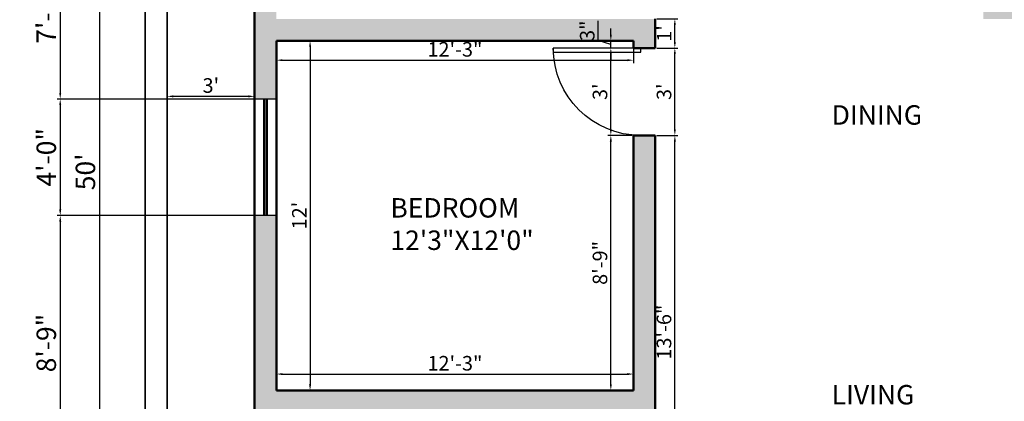
# Model space of a CAD drawing. Units: inches. Extents: x 2442 to 3851, y 589 to 2836.
# Tile 14 of 22: x 2442 to 2847, y 2397 to 2554. Entities that reach past the tile are written whole.
import ezdxf

# ---------------------------------------------------------------- set-up
doc = ezdxf.new("R2010")
doc.units = ezdxf.units.IN
for name, color, linetype, lineweight in [('A-ANNO-DIMS', 2, 'Continuous', 18), ('A-AREA-IDEN', 7, 'Continuous', 18), ('A-DOOR', 4, 'Continuous', 25), ('A-GLAZ', 1, 'Continuous', 25), ('A-WALL', 7, 'Continuous', 50), ('A-WALL-PATT', 8, 'Continuous', 13), ('C-PROP', 7, 'Continuous', 35)]:
    doc.layers.add(name, color=color, linetype=linetype, lineweight=lineweight)
doc.styles.get("Standard").update_dxf_attribs({"font": 'arial.ttf'})
doc.dimstyles.new('ISO-25', dxfattribs={"dimtxt": 8, "dimasz": 2.5, "dimexe": 1.25, "dimexo": 0.625, "dimtad": 1, "dimlunit": 3, "dimtxsty": 'Standard', "dimcen": 2.5, "dimadec": 0, "dimazin": 0, "dimtfac": 1, "dimtmove": 0, "dimatfit": 3, "dimfxl": 1, "dimarcsym": 0})

# ---------------------------------------------------------------- blocks, each defined once
blk = doc.blocks.new('*U23')
for p, q in [((0, 0), (0, -6)), ((36, 0), (36, -6))]:
    blk.add_line(p, q)
blk.add_lwpolyline([(0, 0), (0, 36), (1.75, 36), (1.75, 0)], close=True)
blk.add_arc((0, 0), 36, 0, 90)
blk = doc.blocks.new('*D36')
at = {"layer": 'A-ANNO-DIMS', "color": 0, "lineweight": -2, "transparency": 16777216}
for p, q in [((2492.97, 2791.21), (2473.47, 2791.21)), ((2474.72, 2788.71), (2474.72, 2193.71)), ((2492.97, 2191.21), (2473.47, 2191.21))]:
    blk.add_line(p, q, dxfattribs=at)
at = {"layer": 'A-ANNO-DIMS', "color": 0, "transparency": 16777216}
for points in [[(2474.3, 2788.71), (2475.14, 2788.71), (2474.72, 2791.21)], [(2474.3, 2193.71), (2475.14, 2193.71), (2474.72, 2191.21)]]:
    blk.add_solid(points, dxfattribs=at)
at = {"layer": 'Defpoints', "color": 0, "transparency": 16777216}
for p in [(2493.6, 2791.21), (2474.72, 2191.21), (2493.6, 2191.21)]:
    blk.add_point(p, dxfattribs=at)
at = {"layer": 'A-ANNO-DIMS', "color": 0, "transparency": 16777216, "insert": (2470.01, 2491.21), "char_height": 8, "attachment_point": 5, "rotation": 90}
blk.add_mtext("50'", dxfattribs=at)
blk = doc.blocks.new('*D41')
at = {"layer": 'A-ANNO-DIMS', "color": 0, "lineweight": -2, "transparency": 16777216}
for p, q in [((2502.6, 2521.83), (2502.6, 2523.56)), ((2536.1, 2522.31), (2505.1, 2522.31)), ((2538.6, 2521.83), (2538.6, 2523.56))]:
    blk.add_line(p, q, dxfattribs=at)
at = {"layer": 'A-ANNO-DIMS', "color": 0, "transparency": 16777216}
for points in [[(2505.1, 2522.73), (2505.1, 2521.89), (2502.6, 2522.31)], [(2536.1, 2522.73), (2536.1, 2521.89), (2538.6, 2522.31)]]:
    blk.add_solid(points, dxfattribs=at)
at = {"layer": 'Defpoints', "color": 0, "transparency": 16777216}
for p in [(2502.6, 2522.31), (2502.6, 2521.21), (2538.6, 2521.21)]:
    blk.add_point(p, dxfattribs=at)
at = {"layer": 'A-ANNO-DIMS', "color": 0, "transparency": 16777216, "insert": (2520.6, 2526), "char_height": 6, "attachment_point": 5}
blk.add_mtext("3'", dxfattribs=at)
blk = doc.blocks.new('*D56')
at = {"layer": 'A-ANNO-DIMS', "color": 0, "lineweight": -2, "transparency": 16777216}
for p, q in [((2548.22, 2545.21), (2562.71, 2545.21)), ((2561.46, 2542.71), (2561.46, 2403.71)), ((2548.22, 2401.21), (2562.71, 2401.21))]:
    blk.add_line(p, q, dxfattribs=at)
at = {"layer": 'A-ANNO-DIMS', "color": 0, "transparency": 16777216}
for points in [[(2561.05, 2542.71), (2561.88, 2542.71), (2561.46, 2545.21)], [(2561.05, 2403.71), (2561.88, 2403.71), (2561.46, 2401.21)]]:
    blk.add_solid(points, dxfattribs=at)
at = {"layer": 'Defpoints', "color": 0, "transparency": 16777216}
for p in [(2547.6, 2545.21), (2547.6, 2401.21), (2561.46, 2401.21)]:
    blk.add_point(p, dxfattribs=at)
at = {"layer": 'A-ANNO-DIMS', "color": 0, "transparency": 16777216, "insert": (2557.83, 2473.21), "char_height": 6, "attachment_point": 5, "rotation": 90}
blk.add_mtext("12'", dxfattribs=at)
blk = doc.blocks.new('*D57')
at = {"layer": 'A-ANNO-DIMS', "color": 0, "lineweight": -2, "transparency": 16777216}
for p, q in [((2547.6, 2401.83), (2547.6, 2409.17)), ((2550.1, 2407.92), (2692.1, 2407.92)), ((2694.6, 2401.83), (2694.6, 2409.17))]:
    blk.add_line(p, q, dxfattribs=at)
at = {"layer": 'A-ANNO-DIMS', "color": 0, "transparency": 16777216}
for points in [[(2550.1, 2408.34), (2550.1, 2407.51), (2547.6, 2407.92)], [(2692.1, 2408.34), (2692.1, 2407.51), (2694.6, 2407.92)]]:
    blk.add_solid(points, dxfattribs=at)
at = {"layer": 'Defpoints', "color": 0, "transparency": 16777216}
for p in [(2694.6, 2407.92), (2547.6, 2401.21), (2694.6, 2401.21)]:
    blk.add_point(p, dxfattribs=at)
at = {"layer": 'A-ANNO-DIMS', "color": 0, "transparency": 16777216, "insert": (2621.1, 2411.61), "char_height": 6, "attachment_point": 5}
blk.add_mtext('12\'-3"', dxfattribs=at)
blk = doc.blocks.new('*D73')
at = {"layer": 'A-ANNO-DIMS', "color": 0, "lineweight": -2, "transparency": 16777216}
for p, q in [((2693.97, 2506.21), (2684.03, 2506.21)), ((2685.28, 2403.71), (2685.28, 2503.71)), ((2693.97, 2401.21), (2684.03, 2401.21))]:
    blk.add_line(p, q, dxfattribs=at)
at = {"layer": 'A-ANNO-DIMS', "color": 0, "transparency": 16777216}
for points in [[(2684.87, 2503.71), (2685.7, 2503.71), (2685.28, 2506.21)], [(2684.87, 2403.71), (2685.7, 2403.71), (2685.28, 2401.21)]]:
    blk.add_solid(points, dxfattribs=at)
at = {"layer": 'Defpoints', "color": 0, "transparency": 16777216}
for p in [(2685.28, 2506.21), (2694.6, 2506.21), (2694.6, 2401.21)]:
    blk.add_point(p, dxfattribs=at)
at = {"layer": 'A-ANNO-DIMS', "color": 0, "transparency": 16777216, "insert": (2681.59, 2453.71), "char_height": 6, "attachment_point": 5, "rotation": 90}
blk.add_mtext('8\'-9"', dxfattribs=at)
blk = doc.blocks.new('*D74')
at = {"layer": 'A-ANNO-DIMS', "color": 0, "lineweight": -2, "transparency": 16777216}
for p, q in [((2693.97, 2542.21), (2684.03, 2542.21)), ((2685.28, 2508.71), (2685.28, 2539.71)), ((2693.97, 2506.21), (2684.03, 2506.21))]:
    blk.add_line(p, q, dxfattribs=at)
at = {"layer": 'A-ANNO-DIMS', "color": 0, "transparency": 16777216}
for points in [[(2684.87, 2539.71), (2685.7, 2539.71), (2685.28, 2542.21)], [(2684.87, 2508.71), (2685.7, 2508.71), (2685.28, 2506.21)]]:
    blk.add_solid(points, dxfattribs=at)
at = {"layer": 'Defpoints', "color": 0, "transparency": 16777216}
for p in [(2685.28, 2542.21), (2694.6, 2542.21), (2694.6, 2506.21)]:
    blk.add_point(p, dxfattribs=at)
at = {"layer": 'A-ANNO-DIMS', "color": 0, "transparency": 16777216, "insert": (2681.59, 2524.21), "char_height": 6, "attachment_point": 5, "rotation": 90}
blk.add_mtext("3'", dxfattribs=at)
blk = doc.blocks.new('*D75')
at = {"layer": 'A-ANNO-DIMS', "color": 0, "lineweight": -2, "transparency": 16777216}
for p, q in [((2680.03, 2545.28), (2680.03, 2553.43)), ((2685.28, 2547.71), (2685.28, 2550.21)), ((2685.28, 2543.71), (2680.03, 2545.28)), ((2693.97, 2545.21), (2684.03, 2545.21)), ((2693.97, 2542.21), (2684.03, 2542.21)), ((2685.28, 2542.21), (2685.28, 2545.21)), ((2685.28, 2542.21), (2685.28, 2545.21)), ((2685.28, 2539.71), (2685.28, 2537.21))]:
    blk.add_line(p, q, dxfattribs=at)
at = {"layer": 'A-ANNO-DIMS', "color": 0, "transparency": 16777216}
for points in [[(2684.87, 2547.71), (2685.7, 2547.71), (2685.28, 2545.21)], [(2684.87, 2539.71), (2685.7, 2539.71), (2685.28, 2542.21)]]:
    blk.add_solid(points, dxfattribs=at)
at = {"layer": 'Defpoints', "color": 0, "transparency": 16777216}
for p in [(2685.28, 2545.21), (2694.6, 2545.21), (2694.6, 2542.21)]:
    blk.add_point(p, dxfattribs=at)
at = {"layer": 'A-ANNO-DIMS', "color": 0, "transparency": 16777216, "insert": (2676.34, 2549.35), "char_height": 6, "attachment_point": 5, "rotation": 90}
blk.add_mtext('3"', dxfattribs=at)
blk = doc.blocks.new('*D76')
at = {"layer": 'A-ANNO-DIMS', "color": 0, "lineweight": -2, "transparency": 16777216}
for p, q in [((2547.6, 2544.58), (2547.6, 2535.96)), ((2694.6, 2544.58), (2694.6, 2535.96)), ((2550.1, 2537.21), (2692.1, 2537.21))]:
    blk.add_line(p, q, dxfattribs=at)
at = {"layer": 'A-ANNO-DIMS', "color": 0, "transparency": 16777216}
for points in [[(2550.1, 2537.62), (2550.1, 2536.79), (2547.6, 2537.21)], [(2692.1, 2537.62), (2692.1, 2536.79), (2694.6, 2537.21)]]:
    blk.add_solid(points, dxfattribs=at)
at = {"layer": 'Defpoints', "color": 0, "transparency": 16777216}
for p in [(2547.6, 2545.21), (2694.6, 2545.21), (2694.6, 2537.21)]:
    blk.add_point(p, dxfattribs=at)
at = {"layer": 'A-ANNO-DIMS', "color": 0, "transparency": 16777216, "insert": (2621.1, 2540.9), "char_height": 6, "attachment_point": 5}
blk.add_mtext('12\'-3"', dxfattribs=at)
blk = doc.blocks.new('*D83')
at = {"layer": 'A-ANNO-DIMS', "color": 0, "lineweight": -2, "transparency": 16777216}
for p, q in [((2704.22, 2506.21), (2712.89, 2506.21)), ((2711.64, 2346.71), (2711.64, 2503.71)), ((2704.22, 2344.21), (2712.89, 2344.21))]:
    blk.add_line(p, q, dxfattribs=at)
at = {"layer": 'A-ANNO-DIMS', "color": 0, "transparency": 16777216}
for points in [[(2711.22, 2503.71), (2712.05, 2503.71), (2711.64, 2506.21)], [(2711.22, 2346.71), (2712.05, 2346.71), (2711.64, 2344.21)]]:
    blk.add_solid(points, dxfattribs=at)
at = {"layer": 'Defpoints', "color": 0, "transparency": 16777216}
for p in [(2703.6, 2506.21), (2711.64, 2506.21), (2703.6, 2344.21)]:
    blk.add_point(p, dxfattribs=at)
at = {"layer": 'A-ANNO-DIMS', "color": 0, "transparency": 16777216, "insert": (2707.95, 2425.21), "char_height": 6, "attachment_point": 5, "rotation": 90}
blk.add_mtext('13\'-6"', dxfattribs=at)
blk = doc.blocks.new('*D84')
at = {"layer": 'A-ANNO-DIMS', "color": 0, "lineweight": -2, "transparency": 16777216}
for p, q in [((2704.22, 2542.21), (2712.89, 2542.21)), ((2711.64, 2508.71), (2711.64, 2539.71)), ((2704.22, 2506.21), (2712.89, 2506.21))]:
    blk.add_line(p, q, dxfattribs=at)
at = {"layer": 'A-ANNO-DIMS', "color": 0, "transparency": 16777216}
for points in [[(2711.22, 2539.71), (2712.05, 2539.71), (2711.64, 2542.21)], [(2711.22, 2508.71), (2712.05, 2508.71), (2711.64, 2506.21)]]:
    blk.add_solid(points, dxfattribs=at)
at = {"layer": 'Defpoints', "color": 0, "transparency": 16777216}
for p in [(2703.6, 2542.21), (2711.64, 2542.21), (2703.6, 2506.21)]:
    blk.add_point(p, dxfattribs=at)
at = {"layer": 'A-ANNO-DIMS', "color": 0, "transparency": 16777216, "insert": (2707.95, 2524.21), "char_height": 6, "attachment_point": 5, "rotation": 90}
blk.add_mtext("3'", dxfattribs=at)
blk = doc.blocks.new('*D85')
at = {"layer": 'A-ANNO-DIMS', "color": 0, "lineweight": -2, "transparency": 16777216}
for p, q in [((2704.22, 2554.21), (2712.89, 2554.21)), ((2711.64, 2544.71), (2711.64, 2551.71)), ((2704.22, 2542.21), (2712.89, 2542.21))]:
    blk.add_line(p, q, dxfattribs=at)
at = {"layer": 'A-ANNO-DIMS', "color": 0, "transparency": 16777216}
for points in [[(2711.22, 2551.71), (2712.05, 2551.71), (2711.64, 2554.21)], [(2711.22, 2544.71), (2712.05, 2544.71), (2711.64, 2542.21)]]:
    blk.add_solid(points, dxfattribs=at)
at = {"layer": 'Defpoints', "color": 0, "transparency": 16777216}
for p in [(2703.6, 2554.21), (2711.64, 2554.21), (2703.6, 2542.21)]:
    blk.add_point(p, dxfattribs=at)
at = {"layer": 'A-ANNO-DIMS', "color": 0, "transparency": 16777216, "insert": (2708, 2548.21), "char_height": 6, "attachment_point": 5, "rotation": 90}
blk.add_mtext("1'", dxfattribs=at)
blk = doc.blocks.new('*D200')
at = {"layer": 'A-ANNO-DIMS', "color": 0, "lineweight": -2, "transparency": 16777216}
for p, q in [((2537.97, 2609.71), (2457.35, 2609.71)), ((2458.6, 2607.21), (2458.6, 2523.71)), ((2537.97, 2521.21), (2457.35, 2521.21))]:
    blk.add_line(p, q, dxfattribs=at)
at = {"layer": 'A-ANNO-DIMS', "color": 0, "transparency": 16777216}
for points in [[(2458.18, 2607.21), (2459.02, 2607.21), (2458.6, 2609.71)], [(2458.18, 2523.71), (2459.02, 2523.71), (2458.6, 2521.21)]]:
    blk.add_solid(points, dxfattribs=at)
at = {"layer": 'Defpoints', "color": 0, "transparency": 16777216}
for p in [(2538.6, 2609.71), (2458.6, 2521.21), (2538.6, 2521.21)]:
    blk.add_point(p, dxfattribs=at)
at = {"layer": 'A-ANNO-DIMS', "color": 0, "transparency": 16777216, "insert": (2453.84, 2565.46), "char_height": 8, "attachment_point": 5, "rotation": 90}
blk.add_mtext('7\'-4 1/2"', dxfattribs=at)
blk = doc.blocks.new('*D201')
at = {"layer": 'A-ANNO-DIMS', "color": 0, "lineweight": -2, "transparency": 16777216}
for p, q in [((2537.97, 2521.21), (2457.35, 2521.21)), ((2458.6, 2518.71), (2458.6, 2475.71)), ((2537.97, 2473.21), (2457.35, 2473.21))]:
    blk.add_line(p, q, dxfattribs=at)
at = {"layer": 'A-ANNO-DIMS', "color": 0, "transparency": 16777216}
for points in [[(2458.18, 2518.71), (2459.02, 2518.71), (2458.6, 2521.21)], [(2458.18, 2475.71), (2459.02, 2475.71), (2458.6, 2473.21)]]:
    blk.add_solid(points, dxfattribs=at)
at = {"layer": 'Defpoints', "color": 0, "transparency": 16777216}
for p in [(2538.6, 2521.21), (2458.6, 2473.21), (2538.6, 2473.21)]:
    blk.add_point(p, dxfattribs=at)
at = {"layer": 'A-ANNO-DIMS', "color": 0, "transparency": 16777216, "insert": (2453.89, 2497.21), "char_height": 8, "attachment_point": 5, "rotation": 90}
blk.add_mtext('4\'-0"', dxfattribs=at)
blk = doc.blocks.new('*D202')
at = {"layer": 'A-ANNO-DIMS', "color": 0, "lineweight": -2, "transparency": 16777216}
for p, q in [((2537.97, 2473.21), (2457.35, 2473.21)), ((2458.6, 2470.71), (2458.6, 2370.71)), ((2537.97, 2368.21), (2457.35, 2368.21))]:
    blk.add_line(p, q, dxfattribs=at)
at = {"layer": 'A-ANNO-DIMS', "color": 0, "transparency": 16777216}
for points in [[(2458.18, 2470.71), (2459.02, 2470.71), (2458.6, 2473.21)], [(2458.18, 2370.71), (2459.02, 2370.71), (2458.6, 2368.21)]]:
    blk.add_solid(points, dxfattribs=at)
at = {"layer": 'Defpoints', "color": 0, "transparency": 16777216}
for p in [(2538.6, 2473.21), (2458.6, 2368.21), (2538.6, 2368.21)]:
    blk.add_point(p, dxfattribs=at)
at = {"layer": 'A-ANNO-DIMS', "color": 0, "transparency": 16777216, "insert": (2453.89, 2420.71), "char_height": 8, "attachment_point": 5, "rotation": 90}
blk.add_mtext('8\'-9"', dxfattribs=at)

msp = doc.modelspace()

# ---------------------------------------------------------------- hatches: boundary and pattern name
at = {"layer": 'A-WALL-PATT'}
h = msp.add_hatch(color=256, dxfattribs=at)
h.dxf.hatch_style = 1
h.paths.add_polyline_path([(2640.599, 2713.208), (2640.599, 2719.208), (2640.599, 2722.208), (2538.599, 2722.208), (2538.599, 2657.708), (2547.599, 2657.708), (2547.599, 2713.208)])
h.paths.add_polyline_path([(2700.599, 2737.208), (2730.599, 2737.208), (2730.599, 2746.208), (2700.599, 2746.208), (2700.599, 2782.208), (2691.599, 2782.208), (2691.599, 2722.208), (2670.599, 2722.208), (2670.599, 2719.208), (2670.599, 2713.208), (2691.599, 2713.208), (2691.599, 2608.208), (2799.599, 2608.208), (2799.599, 2614.208), (2799.599, 2617.208), (2700.599, 2617.208)])
h.paths.add_polyline_path([(2838.599, 2737.208), (2838.599, 2617.208), (2835.599, 2617.208), (2835.599, 2614.208), (2835.599, 2608.208), (2838.599, 2608.208), (2838.599, 2554.208), (2850.599, 2554.208), (2850.599, 2560.208), (2850.599, 2563.208), (2847.599, 2563.208), (2847.599, 2737.208), (2850.599, 2737.208), (2850.599, 2746.208), (2796.599, 2746.208), (2796.599, 2737.208)])
h.paths.add_polyline_path([(2898.599, 2746.208), (2898.599, 2737.208), (2967.599, 2737.208), (2967.599, 2746.208)])
h.paths.add_polyline_path([(3048.599, 2746.208), (3015.599, 2746.208), (3015.599, 2737.208), (3039.599, 2737.208), (3039.599, 2665.208), (3048.599, 2665.208)])
h.paths.add_polyline_path([(3039.599, 2611.208), (3039.599, 2605.208), (3048.599, 2605.208), (3048.599, 2617.208), (2946.599, 2617.208), (2946.599, 2611.208)])
h.paths.add_polyline_path([(2961.599, 2563.208), (2961.599, 2581.208), (2955.599, 2581.208), (2955.599, 2563.208), (2895.599, 2563.208), (2895.599, 2611.208), (2916.599, 2611.208), (2916.599, 2617.208), (2889.599, 2617.208), (2889.599, 2563.208), (2886.599, 2563.208), (2886.599, 2554.208), (2937.599, 2554.208), (2937.599, 2536.208), (2943.599, 2536.208), (2943.599, 2554.208), (3039.599, 2554.208), (3039.599, 2548.208), (3048.599, 2548.208), (3048.599, 2569.208), (3039.599, 2569.208), (3039.599, 2563.208)])
h.paths.add_polyline_path([(2538.599, 2521.208), (2547.599, 2521.208), (2547.599, 2545.208), (2694.599, 2545.208), (2694.599, 2542.208), (2697.599, 2542.208), (2703.599, 2542.208), (2703.599, 2554.208), (2547.599, 2554.208), (2547.599, 2609.708), (2538.599, 2609.708)])
h.paths.add_polyline_path([(2538.599, 2368.208), (2547.599, 2368.208), (2547.599, 2392.208), (2694.599, 2392.208), (2694.599, 2344.208), (2703.599, 2344.208), (2703.599, 2506.208), (2697.599, 2506.208), (2694.599, 2506.208), (2694.599, 2401.208), (2547.599, 2401.208), (2547.599, 2473.208), (2538.599, 2473.208)])
h.paths.add_polyline_path([(2547.599, 2287.208), (2553.599, 2287.208), (2553.599, 2293.208), (2553.599, 2296.208), (2547.599, 2296.208), (2547.599, 2320.208), (2538.599, 2320.208), (2538.599, 2191.208), (2547.599, 2191.208)])
h.paths.add_polyline_path([(2703.599, 2296.208), (2670.599, 2296.208), (2670.599, 2287.208), (2694.599, 2287.208), (2694.599, 2248.208), (2733.599, 2248.208), (2733.599, 2257.208), (2703.599, 2257.208)])
h.paths.add_polyline_path([(2593.599, 2287.208), (2604.599, 2287.208), (2604.599, 2296.208), (2593.599, 2296.208)])
h.paths.add_polyline_path([(2799.599, 2248.208), (2799.599, 2257.208), (2775.599, 2257.208), (2775.599, 2248.208)])
h.paths.add_polyline_path([(2892.599, 2248.208), (2892.599, 2287.208), (2883.599, 2287.208), (2883.599, 2257.208), (2865.599, 2257.208), (2865.599, 2248.208)])
h.paths.add_polyline_path([(2883.599, 2353.208), (2892.599, 2353.208), (2892.599, 2392.208), (3048.599, 2392.208), (3048.599, 2426.708), (3039.599, 2426.708), (3039.599, 2401.208), (2892.599, 2401.208), (2892.599, 2461.208), (2883.599, 2461.208)])
h.paths.add_polyline_path([(3039.599, 2474.708), (3048.599, 2474.708), (3048.599, 2512.208), (3039.599, 2512.208), (3039.599, 2506.208), (2937.599, 2506.208), (2937.599, 2500.208), (3039.599, 2500.208)])

# ---------------------------------------------------------------- linework, layer by layer
at = {"layer": 'A-GLAZ'}
for p, q in [((2547.599, 2521.208), (2538.599, 2521.208)), ((2547.599, 2473.208), (2538.599, 2473.208))]:
    msp.add_line(p, q, dxfattribs=at)
at = {"layer": 'A-WALL'}
for p, q in [((2538.599, 2722.208), (2538.599, 2191.208)), ((2703.599, 2542.208), (2703.599, 2554.208)), ((2547.599, 2545.208), (2547.599, 2401.208)), ((2547.599, 2545.208), (2694.599, 2545.208)), ((2694.599, 2542.208), (2694.599, 2545.208)), ((2694.599, 2542.208), (2703.599, 2542.208)), ((2542.599, 2521.208), (2542.599, 2473.208)), ((2543.599, 2521.208), (2543.599, 2473.208)), ((2694.599, 2401.208), (2694.599, 2506.208)), ((2694.599, 2506.208), (2703.599, 2506.208)), ((2703.599, 2344.208), (2703.599, 2506.208)), ((2547.599, 2401.208), (2694.599, 2401.208))]:
    msp.add_line(p, q, dxfattribs=at)
at = {"layer": 'C-PROP'}
for points in [[(3066.599, 2191.208), (3093.599, 2191.208), (3093.599, 2791.208), (2493.599, 2791.208), (2493.599, 2191.208), (2738.599, 2191.208)], [(3066.599, 2200.208), (3084.599, 2200.208), (3084.599, 2782.208), (2502.599, 2782.208), (2502.599, 2200.208), (2538.599, 2200.208)]]:
    msp.add_lwpolyline(points, dxfattribs=at)

# ---------------------------------------------------------------- block references
at = {"layer": 'A-DOOR', "xscale": -1, "rotation": 90}
msp.add_blockref('*U23', (2697.599, 2542.208), dxfattribs=at)

# ---------------------------------------------------------------- texts
at = {"layer": 'A-AREA-IDEN', "char_height": 8, "attachment_point": 1}
for s, insert in [('{\\fTimes New Roman|b0|i0|c0|p18;DINING}', (2776.221, 2518.642)), ('{\\fTimes New Roman|b0|i0|c0|p18;BEDROOM\\P12\'3"X12\'0"}', (2594.523, 2480.39)), ('{\\fTimes New Roman|b0|i0|c0|p18;LIVING\\P15\'0"X17\'0"}', (2776.221, 2403.426))]:
    msp.add_mtext_dynamic_manual_height_columns(s, width=110.76054, gutter_width=12.5, heights=[0], dxfattribs=dict(at, insert=insert))

# ---------------------------------------------------------------- dimensions: what is measured, and where the dimension line sits
at = {"layer": 'A-ANNO-DIMS'}
for base, p1, p2, override, picture, middle in [((2474.719, 2191.208), (2493.599, 2791.208), (2493.599, 2191.208), {"dimclrd": 0, "dimclre": 0, "dimclrt": 0}, '*D36', (2470.009, 2491.208)), ((2458.599, 2521.208), (2538.599, 2609.708), (2538.599, 2521.208), {"dimdec": 1, "dimlfac": 1, "dimrnd": 0, "dimzin": 1, "dimdsep": 46, "dimlunit": 4, "dimfrac": 2}, '*D200', (2453.837, 2565.458)), ((2711.636, 2554.208), (2703.599, 2542.208), (2703.599, 2554.208), {"dimtxt": 6, "dimclrd": 0, "dimclre": 0, "dimclrt": 0, "dimtmove": 1}, '*D85', (2707.998, 2548.208)), ((2685.283, 2545.208), (2694.599, 2542.208), (2694.599, 2545.208), {"dimtxt": 6, "dimclrd": 0, "dimclre": 0, "dimclrt": 0, "dimtmove": 1}, '*D75', (2676.339, 2545.909)), ((2561.464, 2401.208), (2547.599, 2545.208), (2547.599, 2401.208), {"dimtxt": 6, "dimclrd": 0, "dimclre": 0, "dimclrt": 0}, '*D56', (2557.826, 2473.208)), ((2685.283, 2542.208), (2694.599, 2506.208), (2694.599, 2542.208), {"dimtxt": 6, "dimclrd": 0, "dimclre": 0, "dimclrt": 0, "dimtmove": 1}, '*D74', (2681.592, 2524.208)), ((2711.636, 2542.208), (2703.599, 2506.208), (2703.599, 2542.208), {"dimtxt": 6, "dimclrd": 0, "dimclre": 0, "dimclrt": 0, "dimtmove": 1}, '*D84', (2707.945, 2524.208)), ((2458.599, 2473.208), (2538.599, 2521.208), (2538.599, 2473.208), {"dimdec": 1, "dimlfac": 1, "dimrnd": 0, "dimzin": 1, "dimdsep": 46, "dimlunit": 4, "dimfrac": 2}, '*D201', (2453.889, 2497.208)), ((2685.283, 2506.208), (2694.599, 2401.208), (2694.599, 2506.208), {"dimtxt": 6, "dimclrd": 0, "dimclre": 0, "dimclrt": 0}, '*D73', (2681.594, 2453.708)), ((2711.636, 2506.208), (2703.599, 2344.208), (2703.599, 2506.208), {"dimtxt": 6, "dimclrd": 0, "dimclre": 0, "dimclrt": 0, "dimtmove": 1}, '*D83', (2707.945, 2425.208)), ((2458.599, 2368.208), (2538.599, 2473.208), (2538.599, 2368.208), {"dimdec": 1, "dimlfac": 1, "dimrnd": 0, "dimzin": 1, "dimdsep": 46, "dimlunit": 4, "dimfrac": 2}, '*D202', (2453.889, 2420.708))]:
    dim = msp.add_linear_dim(base=base, p1=p1, p2=p2, angle=90, dimstyle='ISO-25', override=override, dxfattribs=at)
    dim.commit()
    dim.dimension.update_dxf_attribs({"geometry": picture, "text_midpoint": middle})
for base, p1, p2, picture, middle in [((2694.599, 2537.208), (2547.599, 2545.208), (2694.599, 2545.208), '*D76', (2621.099, 2540.898)), ((2502.599, 2522.31), (2538.599, 2521.208), (2502.599, 2521.208), '*D41', (2520.599, 2526.001)), ((2694.599, 2407.924), (2547.599, 2401.208), (2694.599, 2401.208), '*D57', (2621.099, 2411.614))]:
    dim = msp.add_linear_dim(base=base, p1=p1, p2=p2, dimstyle='ISO-25', override={"dimtxt": 6, "dimclrd": 0, "dimclre": 0, "dimclrt": 0}, dxfattribs=at)
    dim.commit()
    dim.dimension.update_dxf_attribs({"geometry": picture, "text_midpoint": middle})

doc.saveas('drawing.dxf')
